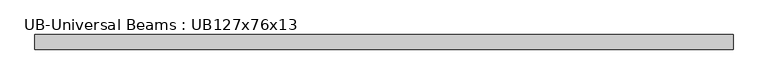
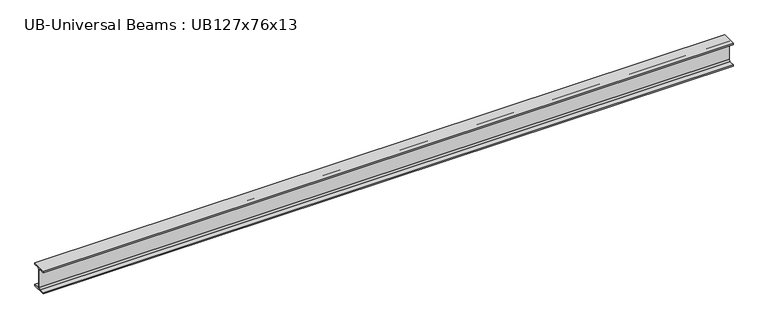
"""IFC4 building model written with IfcOpenShell, lengths in millimetres: member geometry, UB-Universal Beams : UB127x76x13."""

from ifc_helpers import new_model, si_unit, point, frame, frame_2d, origin, place, context, project, spatial, polyline, circle_curve, trimmed, segment, composite_curve, outline, extrude, source, transform, mapped, element, save


def ub_universal_beams_ub127x76x13_03bf5c3b(model_context):
    return source(origin(), model_context, "Body", "SweptSolid", [
        extrude(outline(composite_curve([segment(polyline([(38.0, -55.9), (38.0, -63.5), (-38.0, -63.5), (-38.0, -55.9), (-9.6, -55.9)]), True, "CONTINUOUS"), segment(trimmed(circle_curve(frame_2d((-9.6, -48.3)), 7.6), [point((-9.6, -55.9))], [point((-2.0, -48.3))], True, "CARTESIAN"), True, "CONTINUOUS"), segment(polyline([(-2.0, -48.3), (-2.0, 48.3)]), True, "CONTINUOUS"), segment(trimmed(circle_curve(frame_2d((-9.6, 48.3)), 7.6), [point((-2.0, 48.3))], [point((-9.6, 55.9))], True, "CARTESIAN"), True, "CONTINUOUS"), segment(polyline([(-9.6, 55.9), (-38.0, 55.9), (-38.0, 63.5), (38.0, 63.5), (38.0, 55.9), (9.6, 55.9)]), True, "CONTINUOUS"), segment(trimmed(circle_curve(frame_2d((9.6, 48.3)), 7.6), [point((9.6, 55.9))], [point((2.0, 48.3))], True, "CARTESIAN"), True, "CONTINUOUS"), segment(polyline([(2.0, 48.3), (2.0, -48.3)]), True, "CONTINUOUS"), segment(trimmed(circle_curve(frame_2d((9.6, -48.3)), 7.6), [point((2.0, -48.3))], [point((9.6, -55.9))], True, "CARTESIAN"), True, "CONTINUOUS"), segment(polyline([(9.6, -55.9), (38.0, -55.9)]), True, "CONTINUOUS")], self_intersect=False)), frame((-1597.25, 0.0, 0.0), z_axis=(1.0, 0.0, 0.0), x_axis=(0.0, 1.0, 0.0)), (0.0, 0.0, 1.0), 3626.1),
    ])


if __name__ == "__main__":
    model = new_model("IFC4")
    model_context = context("Model", 3, world=origin())
    ifc_project = project(units=[si_unit("LENGTHUNIT", "METRE", prefix="MILLI")], contexts=[model_context])
    site = spatial("IfcSite", under=ifc_project)
    building = spatial("IfcBuilding", under=site)
    placement = place(None, origin())
    ub_universal_beams_ub127x76x13_shape = ub_universal_beams_ub127x76x13_03bf5c3b(model_context)
    element("IfcMember", 1, ObjectType="UB-Universal Beams : UB127x76x13", at=placement, inside=building, context=model_context, shape_type="MappedRepresentation", body=[
        mapped(ub_universal_beams_ub127x76x13_shape, transform((0.0, 0.0, 0.0), x_axis=(1.0, 0.0, 0.0), y_axis=(0.0, 1.0, 0.0), z_axis=(0.0, 0.0, 1.0))),
    ])
    save(model, "model.ifc")

# Revit data of these elements
# Type "UB-Universal Beams : UB127x76x13"
#   Section Name Key = "UB127X76X13"
#   Width = 7.6 cm
#   Web Thickness = 0.4 cm
#   Web Fillet = 0.76 cm
#   Warping Constant = 2000.0 cm⁶
#   Torsional Moment of Inertia = 2.85 cm⁴
#   Section Area = 16.5 cm²
#   Plastic Modulus weak axis = 22.6 cm³
#   Plastic Modulus strong axis = 84.2 cm³
#   Nominal Weight = 13.00 kgf/m
#   Moment of Inertia weak axis = 55.70 cm⁴
#   Moment of Inertia strong axis = 473.00 cm⁴
#   Height = 12.7 cm
#   Flange Thickness = 0.76 cm
#   Elastic Modulus weak axis = 14.7 cm³
#   Elastic Modulus strong axis = 74.6 cm³
#   Centroid Vertical = 6.35 cm
#   Centroid Horizontal = 3.8 cm
#   Bolt Spacing = 4.0 cm
#   Length [instance default] = 1.5 m
#   Structural Material [instance default] = Metal - Steel 43-275
#   Type Comments = ""
#   Assembly Code = ""
# Element 1 (IfcMember, "UB-Universal Beams : UB127x76x13")
#   Materials on its faces: "Metal - Steel 43-275"
# Materials
#   "Metal - Steel 43-275": class "Metal", colour RGB 247 247 247, transparency 0, Cost = 0
